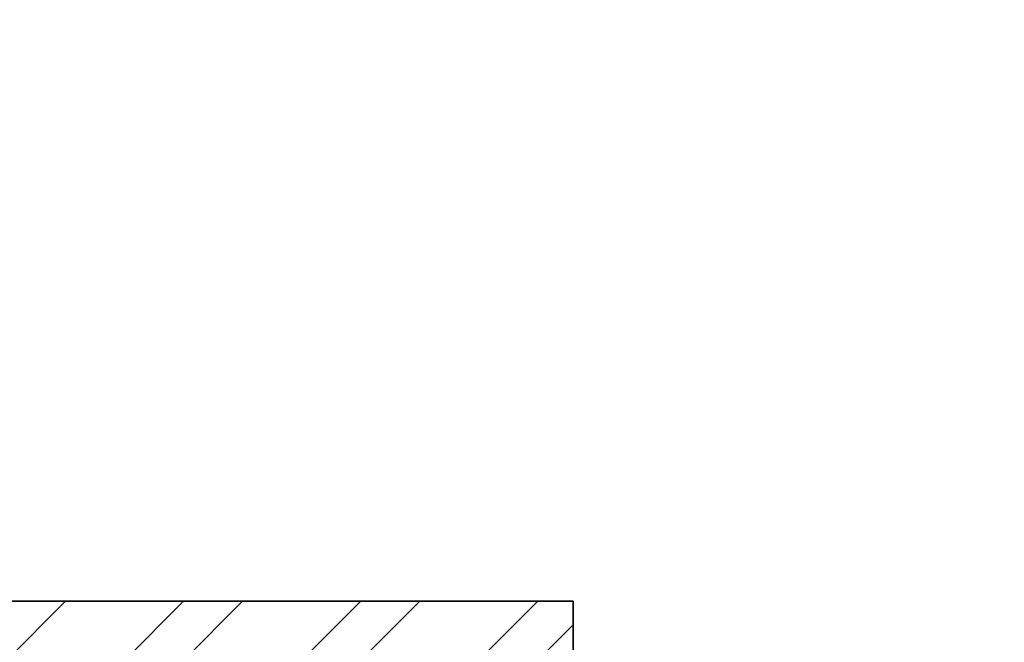
# Model space of a CAD drawing. Units: inches. Extents: x 1885 to 2748, y 783 to 2421.
# Tile 109 of 117: x 2449 to 2524, y 2067 to 2115. Entities that reach past the tile are written whole.
import ezdxf

# ---------------------------------------------------------------- set-up
doc = ezdxf.new("R2010")
doc.units = ezdxf.units.IN
doc.layers.add('A-WALL', color=7, linetype='Continuous', lineweight=35)
doc.layers.add('A-WALL-PATT', color=85, linetype='Continuous', lineweight=13, true_color=0x58ba48)

msp = doc.modelspace()

# ---------------------------------------------------------------- hatches: boundary and pattern name
at = {"layer": 'A-WALL-PATT'}
h = msp.add_hatch(dxfattribs=at)
h.set_pattern_fill('ANSI32', color=256)
h.paths.add_polyline_path([(2007.772, 2318.006), (1980.774, 2318.006), (1980.774, 2281.215), (1985.274, 2281.215), (1985.274, 2313.506), (2007.772, 2313.506), (2007.772, 2315.756)])
h.paths.add_polyline_path([(2094.324, 2318.006), (2067.772, 2318.006), (2067.772, 2313.506), (2094.324, 2313.506), (2094.324, 2315.756)])
h.paths.add_polyline_path([(2131.367, 2315.756), (2131.367, 2318.006), (2131.189, 2318.006), (2112.609, 2318.006), (2112.609, 2313.506), (2117.274, 2313.506), (2117.274, 2255.201), (2121.774, 2255.201), (2121.774, 2313.506), (2131.367, 2313.506)])
h.paths.add_polyline_path([(2190.512, 2318.006), (2155.367, 2318.006), (2155.367, 2313.506), (2169.774, 2313.506), (2169.774, 2229.506), (2121.774, 2229.506), (2121.774, 2233.451), (2119.524, 2233.451), (2117.274, 2233.451), (2117.274, 2201.101), (2121.774, 2201.101), (2121.774, 2225.006), (2169.774, 2225.006), (2169.774, 2165.006), (2306.274, 2165.006), (2306.274, 2066.006), (2310.774, 2066.006), (2344.274, 2066.006), (2486.274, 2066.006), (2486.274, 1886.006), (2483.02, 1886.006), (2483.02, 1881.506), (2486.274, 1881.506), (2486.274, 1880.678), (2490.774, 1880.678), (2490.774, 2070.506), (2344.274, 2070.506), (2310.774, 2070.506), (2310.774, 2165.006), (2310.774, 2173.636), (2308.524, 2173.636), (2306.274, 2173.636), (2306.274, 2169.506), (2174.274, 2169.506), (2174.274, 2313.506), (2190.512, 2313.506), (2190.512, 2315.756)])
h.paths.add_polyline_path([(1985.274, 2221.215), (1980.774, 2221.215), (1980.774, 2165.006), (1992.774, 2165.006), (1992.774, 2141.927), (1997.274, 2141.927), (1997.274, 2165.006), (2117.274, 2165.006), (2117.274, 2163.126), (2121.774, 2163.126), (2121.774, 2172.734), (2119.524, 2172.734), (2117.274, 2172.734), (2117.274, 2169.506), (1985.274, 2169.506)])
h.paths.add_polyline_path([(1997.274, 2105.927), (1992.774, 2105.927), (1992.774, 2070.506), (2016.774, 2070.506), (2016.774, 2059.123), (2019.024, 2059.123), (2021.274, 2059.123), (2021.274, 2070.506), (2117.274, 2070.506), (2117.274, 2022.506), (2114.423, 2022.506), (2114.423, 2018.006), (2123.627, 2018.006), (2123.627, 2020.256), (2123.627, 2022.506), (2121.774, 2022.506), (2121.774, 2142.587), (2119.524, 2142.587), (2117.274, 2142.587), (2117.274, 2075.006), (1997.274, 2075.006)])
h.paths.add_polyline_path([(2092.029, 2020.256), (2092.029, 2022.506), (2021.274, 2022.506), (2021.274, 2035.123), (2016.774, 2035.123), (2016.774, 2018.006), (2016.774, 1978.784), (2021.274, 1978.784), (2021.274, 2018.006), (2092.029, 2018.006)])
h.paths.add_polyline_path([(2260.938, 2022.506), (2153.105, 2022.506), (2153.105, 2020.256), (2153.105, 2018.006), (2155.274, 2018.006), (2155.274, 1886.006), (2107.629, 1886.006), (2107.629, 1881.506), (2182.911, 1881.506), (2182.911, 1883.756), (2182.911, 1886.006), (2159.774, 1886.006), (2159.774, 2018.006), (2260.938, 2018.006), (2260.938, 2020.256)])
h.paths.add_polyline_path([(2047.629, 1883.756), (2047.629, 1886.006), (2021.274, 1886.006), (2021.274, 1918.784), (2019.024, 1918.784), (2016.774, 1918.784), (2016.774, 1881.506), (2047.629, 1881.506)])
h.paths.add_polyline_path([(2306.361, 1883.756), (2306.361, 1886.006), (2296.274, 1886.006), (2296.274, 1982.006), (2316.535, 1982.006), (2316.535, 1984.256), (2316.535, 1986.506), (2296.274, 1986.506), (2296.274, 2022.506), (2289.276, 2022.506), (2289.276, 2018.006), (2291.774, 2018.006), (2291.774, 1886.006), (2242.911, 1886.006), (2242.911, 1881.506), (2306.361, 1881.506)], flags=17)
h.paths.add_polyline_path([(1985.274, 1843.006), (2021.6, 1843.006), (2021.534, 1845.441), (2021.477, 1847.506), (1980.774, 1847.506), (1980.774, 1809.446), (1985.274, 1809.446)])
h.paths.add_polyline_path([(2131.482, 1845.256), (2131.482, 1847.506), (2081.534, 1847.506), (2081.534, 1843.006), (2117.274, 1843.006), (2117.274, 1784.147), (2119.524, 1784.147), (2121.774, 1784.147), (2121.774, 1843.006), (2131.482, 1843.006)])
h.paths.add_polyline_path([(2203.886, 1847.506), (2155.482, 1847.506), (2155.482, 1843.006), (2169.774, 1843.006), (2169.774, 1759.006), (2121.774, 1759.006), (2121.774, 1761.457), (2117.274, 1761.457), (2117.274, 1730.429), (2121.774, 1730.429), (2121.774, 1754.506), (2177.421, 1754.506), (2177.421, 1756.756), (2177.421, 1759.006), (2174.274, 1759.006), (2174.274, 1843.006), (2203.886, 1843.006)])
h.paths.add_polyline_path([(2335.554, 1845.256), (2335.554, 1847.506), (2239.886, 1847.506), (2239.886, 1843.006), (2306.274, 1843.006), (2306.274, 1759.006), (2199.486, 1759.006), (2199.486, 1754.506), (2310.774, 1754.506), (2310.774, 1843.006), (2335.554, 1843.006)])
h.paths.add_polyline_path([(2348.774, 2022.506), (2344.274, 2022.506), (2344.274, 1986.506), (2341.681, 1986.506), (2341.681, 1982.006), (2344.274, 1982.006), (2344.274, 1886.006), (2330.361, 1886.006), (2330.361, 1881.506), (2361.627, 1881.506), (2361.627, 1883.756), (2361.627, 1886.006), (2348.774, 1886.006)], flags=17)
h.paths.add_polyline_path([(2283.251, 2315.756), (2283.251, 2318.006), (2238.512, 2318.006), (2238.512, 2313.506), (2283.251, 2313.506)], flags=17)
h.paths.add_polyline_path([(2363.274, 2348.006), (2388.677, 2348.006), (2388.677, 2350.256), (2388.677, 2352.506), (2358.774, 2352.506), (2358.774, 2348.006), (2358.774, 2318.006), (2344.481, 2318.006), (2344.481, 2313.506), (2358.774, 2313.506), (2358.774, 2229.506), (2310.774, 2229.506), (2310.774, 2231.952), (2306.274, 2231.952), (2306.274, 2205.611), (2310.774, 2205.611), (2310.774, 2225.006), (2358.774, 2225.006), (2358.774, 2211.506), (2452.329, 2211.506), (2452.329, 2213.756), (2452.329, 2216.006), (2363.274, 2216.006), (2363.274, 2318.006)])
h.paths.add_polyline_path([(2310.774, 2313.506), (2320.481, 2313.506), (2320.481, 2315.756), (2320.481, 2318.006), (2302.728, 2318.006), (2302.728, 2313.506), (2306.274, 2313.506), (2306.274, 2251.076), (2310.774, 2251.076)], flags=17)
h.paths.add_polyline_path([(2490.774, 2352.506), (2486.274, 2352.506), (2448.677, 2352.506), (2448.677, 2348.006), (2486.274, 2348.006), (2486.274, 2318.006), (2486.274, 2216.006), (2481.78, 2216.006), (2481.78, 2211.506), (2486.274, 2211.506), (2486.274, 2165.006), (2493.289, 2165.006), (2493.289, 2167.256), (2493.289, 2169.506), (2490.774, 2169.506), (2490.774, 2313.506), (2494.429, 2313.506), (2494.429, 2318.006), (2490.774, 2318.006)])
h.paths.add_polyline_path([(2534.653, 2318.006), (2515.691, 2318.006), (2515.691, 2313.506), (2534.653, 2313.506), (2534.653, 2315.756)])
h.paths.add_polyline_path([(2618.274, 2318.006), (2594.653, 2318.006), (2594.653, 2313.506), (2613.774, 2313.506), (2613.774, 2281.706), (2618.274, 2281.706)])
h.paths.add_polyline_path([(2618.274, 2221.706), (2613.774, 2221.706), (2613.774, 2169.506), (2554.019, 2169.506), (2554.019, 2165.006), (2613.774, 2165.006), (2613.774, 2152.878), (2618.274, 2152.878)])
h.paths.add_polyline_path([(2618.274, 2128.878), (2616.024, 2128.878), (2613.774, 2128.878), (2613.774, 2117.006), (2529.774, 2117.006), (2529.774, 2165.006), (2532.848, 2165.006), (2532.848, 2169.506), (2522.867, 2169.506), (2522.867, 2165.006), (2525.274, 2165.006), (2525.274, 2117.006), (2525.274, 2112.506), (2525.274, 2108.576), (2529.774, 2108.576), (2529.774, 2112.506), (2613.774, 2112.506), (2613.774, 2080.19), (2618.274, 2080.19)])
h.paths.add_polyline_path([(2618.274, 2044.19), (2616.024, 2044.19), (2613.774, 2044.19), (2613.774, 2015.506), (2529.774, 2015.506), (2529.774, 2088.582), (2527.524, 2088.582), (2525.274, 2088.582), (2525.274, 2011.006), (2613.774, 2011.006), (2613.774, 1956.755), (2618.274, 1956.755)])
h.paths.add_polyline_path([(2618.274, 1881.506), (2618.274, 1896.755), (2613.774, 1896.755), (2613.774, 1881.506), (2613.774, 1847.506), (2592.715, 1847.506), (2592.715, 1843.006), (2613.774, 1843.006), (2613.774, 1765.006), (2613.774, 1760.506), (2609.621, 1760.506), (2609.621, 1756.006), (2613.774, 1756.006), (2613.774, 1660.006), (2608.544, 1660.006), (2608.544, 1655.506), (2613.774, 1655.506), (2613.774, 1508.158), (2618.274, 1508.158)])
h.paths.add_polyline_path([(2565.774, 1843.006), (2568.997, 1843.006), (2568.997, 1847.506), (2490.774, 1847.506), (2490.774, 1849.7), (2488.524, 1849.7), (2486.274, 1849.7), (2486.274, 1847.506), (2477.274, 1847.506), (2477.274, 1838.506), (2477.274, 1821.493), (2486.274, 1821.493), (2486.274, 1838.506), (2561.274, 1838.506), (2561.274, 1765.006), (2486.274, 1765.006), (2486.274, 1786.157), (2477.274, 1786.157), (2477.274, 1765.006), (2477.274, 1756.006), (2486.274, 1756.006), (2565.774, 1756.006), (2585.621, 1756.006), (2585.621, 1758.256), (2585.621, 1760.506), (2565.774, 1760.506), (2565.774, 1765.006)])
h.paths.add_polyline_path([(2486.274, 1651.006), (2561.274, 1651.006), (2561.274, 1567.006), (2486.274, 1567.006), (2486.274, 1591.321), (2477.274, 1591.321), (2477.274, 1567.006), (2477.274, 1558.006), (2477.274, 1555.439), (2481.774, 1555.439), (2481.774, 1558.006), (2568.653, 1558.006), (2568.653, 1560.256), (2568.653, 1562.506), (2565.774, 1562.506), (2565.774, 1655.506), (2584.544, 1655.506), (2584.544, 1657.756), (2584.544, 1660.006), (2565.774, 1660.006), (2486.274, 1660.006), (2477.274, 1660.006), (2477.274, 1651.006), (2477.274, 1632.989), (2486.274, 1632.989)])
h.paths.add_polyline_path([(2449.967, 1883.756), (2449.967, 1886.006), (2421.627, 1886.006), (2421.627, 1881.506), (2449.967, 1881.506)], flags=17)
h.paths.add_polyline_path([(2447.274, 1847.506), (2395.554, 1847.506), (2395.554, 1843.006), (2442.774, 1843.006), (2442.774, 1809.27), (2447.274, 1809.27)])
h.paths.add_polyline_path([(1985.274, 1749.446), (1980.774, 1749.446), (1980.774, 1694.504), (1985.274, 1694.504), (1985.274, 1694.506), (1986.897, 1694.506), (1986.897, 1697.78), (1986.897, 1699.006), (1985.274, 1699.006)])
h.paths.add_polyline_path([(2152.774, 1699.006), (2121.774, 1699.006), (2121.774, 1703.668), (2119.524, 1703.668), (2117.274, 1703.668), (2117.274, 1699.006), (2009.219, 1699.006), (2009.219, 1694.506), (2148.274, 1694.506), (2148.274, 1692.631), (2152.774, 1692.631)])
h.paths.add_polyline_path([(2016.274, 1694.506), (2011.774, 1694.506), (2011.774, 1558.006), (2040.806, 1558.006), (2040.806, 1560.256), (2040.806, 1562.506), (2016.274, 1562.506)])
h.paths.add_polyline_path([(2152.774, 1663.017), (2150.524, 1663.017), (2148.274, 1663.017), (2148.274, 1562.506), (2100.806, 1562.506), (2100.806, 1558.006), (2165.119, 1558.006), (2165.119, 1560.256), (2165.119, 1562.506), (2152.774, 1562.506), (2152.774, 1610.506), (2224.774, 1610.506), (2224.774, 1607.99), (2229.274, 1607.99), (2229.274, 1615.006), (2152.774, 1615.006)])
h.paths.add_polyline_path([(2238.613, 1560.256), (2238.613, 1562.506), (2229.274, 1562.506), (2229.274, 1588.756), (2227.024, 1588.763), (2224.774, 1588.771), (2224.774, 1562.506), (2189.119, 1562.506), (2189.119, 1558.006), (2238.613, 1558.006)])
h.paths.add_polyline_path([(2336.024, 1560.256), (2336.024, 1562.506), (2310.774, 1562.506), (2310.774, 1656.347), (2308.524, 1656.347), (2306.274, 1656.347), (2306.274, 1562.506), (2286.613, 1562.506), (2286.613, 1558.006), (2336.024, 1558.006)])
h.paths.add_polyline_path([(2447.274, 1690.968), (2445.024, 1690.968), (2442.774, 1690.968), (2442.774, 1687.006), (2306.274, 1687.006), (2306.274, 1680.75), (2310.774, 1680.75), (2310.774, 1682.506), (2442.774, 1682.506), (2442.774, 1562.506), (2396.024, 1562.506), (2396.024, 1558.006), (2447.274, 1558.006)])
h.paths.add_polyline_path([(2447.274, 1749.27), (2445.024, 1749.27), (2442.774, 1749.27), (2442.774, 1717.232), (2447.274, 1717.232)])
h.paths.add_polyline_path([(2044.674, 1521.756), (2044.674, 1524.006), (2007.274, 1524.006), (2007.274, 1503.49), (2009.524, 1503.49), (2011.774, 1503.49), (2011.774, 1519.506), (2044.674, 1519.506)])
h.paths.add_polyline_path([(2177.969, 1521.756), (2177.969, 1524.006), (2104.674, 1524.006), (2104.674, 1519.506), (2145.774, 1519.506), (2145.774, 1387.506), (2143.37, 1387.506), (2143.37, 1383.006), (2251.585, 1383.006), (2251.585, 1385.256), (2251.585, 1387.506), (2150.274, 1387.506), (2150.274, 1519.506), (2177.969, 1519.506)])
h.paths.add_polyline_path([(2298.704, 1524.006), (2237.969, 1524.006), (2237.969, 1519.506), (2282.274, 1519.506), (2282.274, 1387.506), (2279.683, 1387.506), (2279.683, 1383.006), (2286.774, 1383.006), (2286.774, 1419.006), (2312.451, 1419.006), (2312.451, 1421.256), (2312.451, 1423.506), (2286.774, 1423.506), (2286.774, 1519.506), (2298.704, 1519.506), (2298.704, 1521.722)], flags=17)
h.paths.add_polyline_path([(2361.897, 1521.756), (2361.897, 1524.006), (2322.704, 1524.006), (2322.704, 1519.506), (2334.774, 1519.506), (2334.774, 1423.506), (2331.93, 1423.506), (2331.93, 1419.006), (2334.774, 1419.006), (2334.774, 1387.506), (2334.774, 1383.228), (2339.274, 1383.228), (2339.274, 1387.506), (2339.274, 1519.506), (2361.897, 1519.506)], flags=17)
h.paths.add_polyline_path([(2447.274, 1521.756), (2447.274, 1524.006), (2421.897, 1524.006), (2421.897, 1519.506), (2447.274, 1519.506)], flags=17)
h.paths.add_polyline_path([(2481.774, 1529.6), (2479.524, 1529.6), (2477.274, 1529.6), (2477.274, 1524.006), (2474.489, 1524.006), (2474.489, 1519.506), (2477.274, 1519.506), (2477.274, 1334.506), (2296.774, 1334.506), (2296.774, 1240.506), (2160.274, 1240.506), (2160.274, 1180.506), (2112.274, 1180.506), (2112.274, 1207.692), (2110.024, 1207.692), (2107.774, 1207.692), (2107.774, 1171.609), (2112.274, 1171.609), (2112.274, 1176.006), (2160.274, 1176.006), (2160.274, 1092.006), (2144.221, 1092.006), (2144.221, 1087.506), (2189.497, 1087.506), (2189.497, 1089.756), (2189.497, 1092.006), (2164.774, 1092.006), (2164.774, 1236.006), (2296.774, 1236.006), (2296.774, 1231.912), (2301.274, 1231.912), (2301.274, 1330.006), (2481.774, 1330.006), (2481.774, 1387.506)])
h.paths.add_polyline_path([(2618.274, 1448.158), (2613.774, 1448.158), (2613.774, 1382.506), (2529.774, 1382.506), (2525.274, 1382.506), (2525.274, 1307.062), (2529.774, 1307.062), (2529.774, 1378.006), (2613.774, 1378.006), (2613.774, 1354.988), (2618.274, 1354.988)])
h.paths.add_polyline_path([(2618.274, 1318.988), (2613.774, 1318.988), (2613.774, 1281.006), (2529.774, 1281.006), (2529.774, 1283.786), (2527.524, 1283.786), (2525.274, 1283.786), (2525.274, 1228.506), (2516.794, 1228.506), (2516.794, 1224.006), (2533.484, 1224.006), (2533.484, 1226.256), (2533.484, 1228.506), (2529.774, 1228.506), (2529.774, 1276.506), (2613.774, 1276.506), (2613.774, 1266.02), (2618.274, 1266.02)])
h.paths.add_polyline_path([(2618.274, 1134.964), (2613.774, 1134.964), (2613.774, 1092.006), (2594.545, 1092.006), (2594.545, 1087.506), (2618.274, 1087.506)])
h.paths.add_polyline_path([(2534.545, 1092.006), (2509.765, 1092.006), (2509.765, 1087.506), (2534.545, 1087.506), (2534.545, 1089.756)])
h.paths.add_polyline_path([(2481.274, 1224.006), (2484.117, 1224.006), (2484.117, 1226.256), (2484.117, 1228.506), (2476.774, 1228.506), (2476.774, 1198.506), (2471.61, 1198.506), (2471.61, 1194.006), (2476.774, 1194.006), (2476.774, 1062.006), (2436.894, 1062.006), (2436.894, 1057.506), (2476.774, 1057.506), (2481.274, 1057.506), (2481.274, 1062.006), (2481.274, 1087.506), (2485.354, 1087.506), (2485.354, 1089.756), (2485.354, 1092.006), (2481.274, 1092.006), (2481.274, 1117.506)])
h.paths.add_polyline_path([(2439.898, 1198.506), (2349.274, 1198.506), (2349.274, 1194.006), (2349.274, 1180.506), (2301.274, 1180.506), (2301.274, 1201.896), (2299.024, 1201.896), (2296.774, 1201.896), (2296.774, 1172.335), (2299.024, 1172.335), (2301.274, 1172.335), (2301.274, 1176.006), (2349.274, 1176.006), (2349.274, 1092.006), (2334.452, 1092.006), (2334.452, 1087.506), (2349.274, 1087.506), (2349.274, 1057.506), (2353.774, 1057.506), (2376.894, 1057.506), (2376.894, 1059.756), (2376.894, 1062.006), (2353.774, 1062.006), (2353.774, 1087.506), (2353.774, 1180.506), (2353.774, 1194.006), (2439.898, 1194.006), (2439.898, 1196.256)])
h.paths.add_polyline_path([(2270.596, 1089.756), (2270.596, 1092.006), (2249.497, 1092.006), (2249.497, 1087.506), (2270.596, 1087.506)], flags=17)
h.paths.add_polyline_path([(2310.452, 1092.006), (2301.274, 1092.006), (2301.274, 1153.292), (2296.774, 1153.292), (2296.774, 1092.006), (2293.786, 1092.006), (2293.786, 1087.506), (2310.452, 1087.506), (2310.452, 1089.756)], flags=17)
h.paths.add_polyline_path([(2112.274, 1150.328), (2110.024, 1150.328), (2107.774, 1150.328), (2107.774, 1092.006), (2104.465, 1092.006), (2104.465, 1087.506), (2120.221, 1087.506), (2120.221, 1089.756), (2120.221, 1092.006), (2112.274, 1092.006)])
h.paths.add_polyline_path([(2082.172, 1092.006), (2058.144, 1092.006), (2058.144, 1087.506), (2082.172, 1087.506), (2082.172, 1089.756)])
h.paths.add_polyline_path([(1975.774, 1145.638), (1971.274, 1145.638), (1971.274, 1087.506), (1980.774, 1087.506), (1998.144, 1087.506), (1998.144, 1089.756), (1998.144, 1092.006), (1985.274, 1092.006), (1975.774, 1092.006)])
h.paths.add_polyline_path([(2112.274, 1244.385), (2110.024, 1244.385), (2107.774, 1244.385), (2107.774, 1240.506), (1992.274, 1240.506), (1992.274, 1271.008), (1987.774, 1271.008), (1987.774, 1240.506), (1980.774, 1240.506), (1975.774, 1240.506), (1971.274, 1240.506), (1971.274, 1205.638), (1975.774, 1205.638), (1975.774, 1236.006), (2107.774, 1236.006), (2107.774, 1233.444), (2112.274, 1233.444), (2112.274, 1236.006)])
h.paths.add_polyline_path([(2112.274, 1383.006), (2114.783, 1383.006), (2114.783, 1385.256), (2114.783, 1387.506), (2102.476, 1387.506), (2102.476, 1383.006), (2107.774, 1383.006), (2107.774, 1335.006), (2011.774, 1335.006), (2011.774, 1349.939), (2007.274, 1349.939), (2007.274, 1335.006), (1987.774, 1335.006), (1987.774, 1330.506), (1987.774, 1307.008), (1992.274, 1307.008), (1992.274, 1330.506), (2007.274, 1330.506), (2107.774, 1330.506), (2107.774, 1264.711), (2112.274, 1264.711)])
h.paths.add_polyline_path([(2077.857, 1387.506), (2011.774, 1387.506), (2011.774, 1390.036), (2009.524, 1390.036), (2007.274, 1390.036), (2007.274, 1373.939), (2011.774, 1373.939), (2011.774, 1383.006), (2077.857, 1383.006)])
h.paths.add_polyline_path([(2011.774, 1443.49), (2007.274, 1443.49), (2007.274, 1410.248), (2011.774, 1410.248)])

# ---------------------------------------------------------------- linework, layer by layer
at = {"layer": 'A-WALL'}
for q in [(2344.274, 2070.506), (2490.774, 1879.236)]:
    msp.add_line((2490.774, 2070.506), q, dxfattribs=at)

doc.saveas('drawing.dxf')
